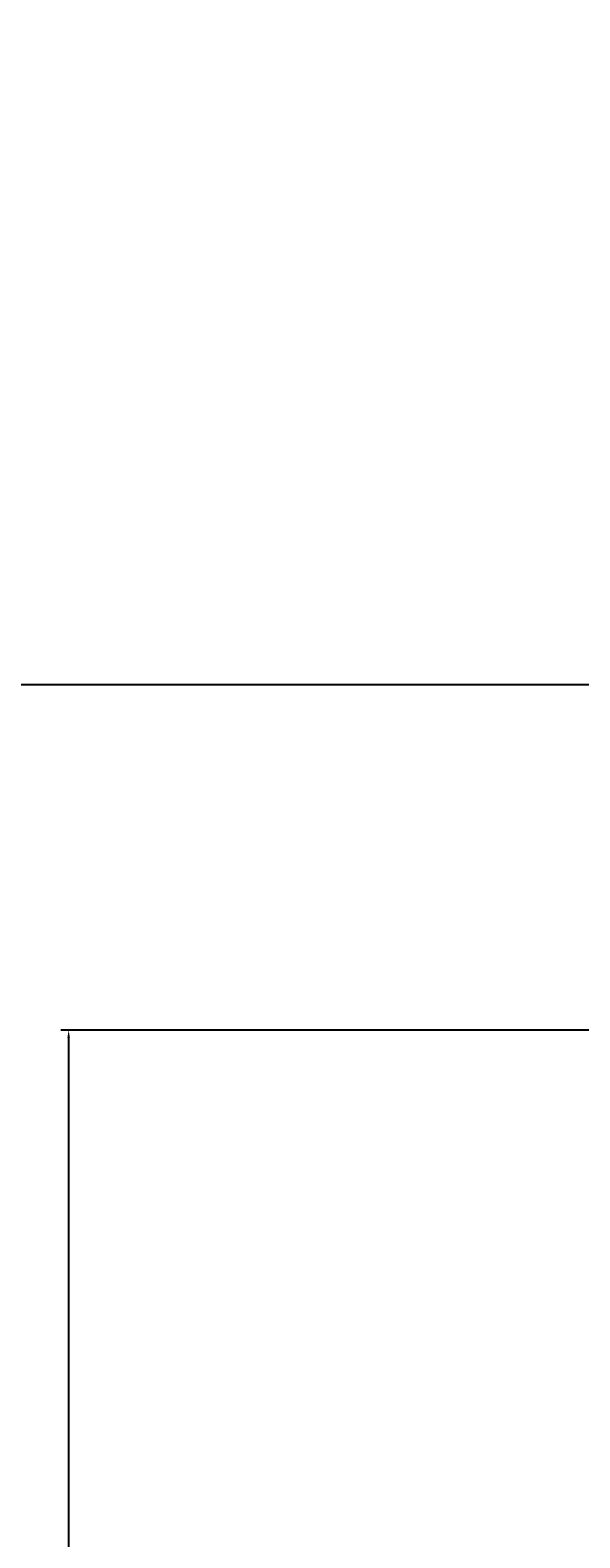
# Model space of a CAD drawing. Units: inches. Extents: x -301 to 715, y -607 to 364.
# Tile 39 of 141: x 121 to 134, y -405 to -370. Entities that reach past the tile are written whole.
import ezdxf

# ---------------------------------------------------------------- set-up
doc = ezdxf.new("R2010")
doc.units = ezdxf.units.IN
doc.header["$MEASUREMENT"] = 0
doc.layers.add('A-ANNO-DIMS', color=2, linetype='Continuous', lineweight=18)
doc.styles.get("Standard").update_dxf_attribs({"font": 'arial.ttf'})
doc.dimstyles.get("Standard").update_dxf_attribs({"dimtxt": 0.18, "dimasz": 0.18, "dimexe": 0.18, "dimexo": 0.0625, "dimgap": 0.09, "dimtad": 0, "dimtih": 1, "dimtoh": 1, "dimdec": 1, "dimzin": 0, "dimdsep": 46, "dimlunit": 4, "dimtxsty": 'Standard', "dimcen": 0.09, "dimclrd": 3, "dimclre": 4, "dimclrt": 6, "dimadec": 0, "dimazin": 0, "dimtfac": 1, "dimtdec": 1, "dimtofl": 0, "dimtmove": 0, "dimatfit": 3, "dimfxl": 1, "dimtfill": 2, "dimtfillclr": 51, "dimtolj": 1, "dimtzin": 0, "dimarcsym": 0})

# ---------------------------------------------------------------- blocks, each defined once
blk = doc.blocks.new('*D176')
at = {"layer": 'A-ANNO-DIMS', "color": 4, "lineweight": -2, "transparency": 16777216}
for p, q in [((148.28, -324.477), (215.605, -324.477)), ((-15.22, -540.477), (215.605, -540.477))]:
    blk.add_line(p, q, dxfattribs=at)
at = {"layer": 'A-ANNO-DIMS', "color": 3, "lineweight": -2, "transparency": 16777216}
for p, q in [((215.425, -324.657), (215.425, -432.296)), ((215.425, -540.297), (215.425, -432.659))]:
    blk.add_line(p, q, dxfattribs=at)
at = {"layer": 'A-ANNO-DIMS', "color": 3, "transparency": 16777216}
for points in [[(215.395, -324.657), (215.455, -324.657), (215.425, -324.477)], [(215.395, -540.297), (215.455, -540.297), (215.425, -540.477)]]:
    blk.add_solid(points, dxfattribs=at)
at = {"layer": 'Defpoints', "color": 0, "transparency": 16777216}
for p in [(148.218, -324.477), (-15.282, -540.477), (215.425, -540.477)]:
    blk.add_point(p, dxfattribs=at)
at = {"layer": 'A-ANNO-DIMS', "color": 6, "transparency": 16777216, "insert": (215.425, -432.477), "char_height": 0.18, "attachment_point": 5, "bg_fill": 1, "box_fill_scale": 1.25, "bg_fill_color": 51, "bg_fill_transparency": 0}
blk.add_mtext('\\A1;18\'-0"', dxfattribs=at)
blk = doc.blocks.new('*D187')
at = {"layer": 'A-ANNO-DIMS', "color": 4, "lineweight": -2, "transparency": 16777216}
for p, q in [((139.674, -385.477), (-266.112, -385.477)), ((143.155, -439.477), (-266.112, -439.477))]:
    blk.add_line(p, q, dxfattribs=at)
at = {"layer": 'A-ANNO-DIMS', "color": 3, "lineweight": -2, "transparency": 16777216}
for p, q in [((-265.932, -385.657), (-265.932, -412.296)), ((-265.932, -439.297), (-265.932, -412.659))]:
    blk.add_line(p, q, dxfattribs=at)
at = {"layer": 'A-ANNO-DIMS', "color": 3, "transparency": 16777216}
for points in [[(-265.962, -385.657), (-265.902, -385.657), (-265.932, -385.477)], [(-265.962, -439.297), (-265.902, -439.297), (-265.932, -439.477)]]:
    blk.add_solid(points, dxfattribs=at)
at = {"layer": 'Defpoints', "color": 0, "transparency": 16777216}
for p in [(-265.932, -385.477), (139.737, -385.477), (143.218, -439.477)]:
    blk.add_point(p, dxfattribs=at)
at = {"layer": 'A-ANNO-DIMS', "color": 6, "transparency": 16777216, "insert": (-265.932, -412.477), "char_height": 0.18, "attachment_point": 5, "bg_fill": 1, "box_fill_scale": 1.25, "bg_fill_color": 51, "bg_fill_transparency": 0}
blk.add_mtext('\\A1;4\'-6"', dxfattribs=at)
blk = doc.blocks.new('*D200')
at = {"layer": 'A-ANNO-DIMS', "color": 4, "lineweight": -2, "transparency": 16777216}
for p, q in [((412.955, -393.552), (121.926, -393.552)), ((412.955, -489.552), (121.926, -489.552))]:
    blk.add_line(p, q, dxfattribs=at)
at = {"layer": 'A-ANNO-DIMS', "color": 3, "lineweight": -2, "transparency": 16777216}
for p, q in [((122.106, -393.732), (122.106, -441.371)), ((122.106, -489.372), (122.106, -441.734))]:
    blk.add_line(p, q, dxfattribs=at)
at = {"layer": 'A-ANNO-DIMS', "color": 3, "transparency": 16777216}
for points in [[(122.076, -393.732), (122.136, -393.732), (122.106, -393.552)], [(122.076, -489.372), (122.136, -489.372), (122.106, -489.552)]]:
    blk.add_solid(points, dxfattribs=at)
at = {"layer": 'Defpoints', "color": 0, "transparency": 16777216}
for p in [(122.106, -393.552), (413.018, -393.552), (413.018, -489.552)]:
    blk.add_point(p, dxfattribs=at)
at = {"layer": 'A-ANNO-DIMS', "color": 6, "transparency": 16777216, "insert": (122.106, -441.552), "char_height": 0.18, "attachment_point": 5, "bg_fill": 1, "box_fill_scale": 1.25, "bg_fill_color": 51, "bg_fill_transparency": 0}
blk.add_mtext('\\A1;8\'-0"', dxfattribs=at)

msp = doc.modelspace()

# ---------------------------------------------------------------- dimensions: what is measured, and where the dimension line sits
at = {"layer": 'A-ANNO-DIMS'}
for base, p1, p2, picture, middle in [((215.425, -540.477), (148.218, -324.477), (-15.282, -540.477), '*D176', (215.425, -432.477)), ((-265.932, -385.477), (143.218, -439.477), (139.737, -385.477), '*D187', (-265.932, -412.477)), ((122.106, -393.552), (413.018, -489.552), (413.018, -393.552), '*D200', (122.106, -441.552))]:
    dim = msp.add_linear_dim(base=base, p1=p1, p2=p2, angle=90, dimstyle='Standard', override={"dimdec": 1, "dimlfac": 1, "dimrnd": 0, "dimzin": 1, "dimdsep": 46, "dimlunit": 4, "dimfrac": 2}, dxfattribs=at)
    dim.commit()
    dim.dimension.update_dxf_attribs({"geometry": picture, "text_midpoint": middle})

doc.saveas('drawing.dxf')
